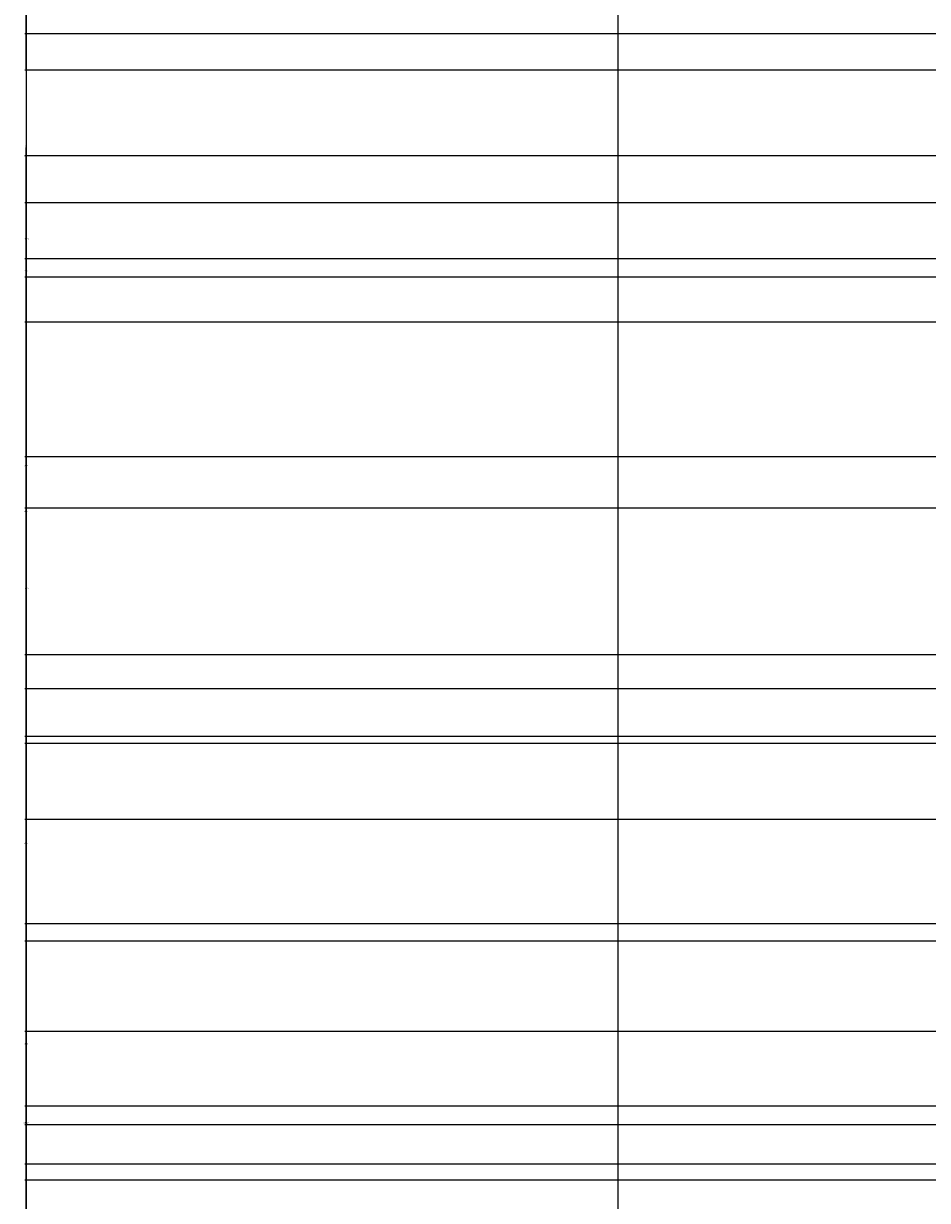
# Model space of a CAD drawing. Units: inches. Extents: x 818 to 1898, y 976 to 2364.
# Tile 57 of 96: x 818 to 950, y 1873 to 2046. Entities that reach past the tile are written whole.
import ezdxf

# ---------------------------------------------------------------- set-up
doc = ezdxf.new("R2010")
doc.units = ezdxf.units.IN
doc.header["$LTSCALE"] = 5
doc.header["$MEASUREMENT"] = 0
doc.layers.add('A-ANNO-DIMS', color=2, linetype='Continuous', lineweight=18)
doc.styles.get("Standard").update_dxf_attribs({"font": 'arial.ttf'})
doc.dimstyles.get("Standard").update_dxf_attribs({"dimtxt": 0.18, "dimasz": 0.18, "dimexe": 0.18, "dimexo": 0.0625, "dimgap": 0.09, "dimtad": 0, "dimtih": 1, "dimtoh": 1, "dimdec": 4, "dimzin": 0, "dimdsep": 46, "dimtxsty": 'Standard', "dimcen": 0.09, "dimadec": 0, "dimazin": 0, "dimtfac": 1, "dimtdec": 4, "dimtofl": 0, "dimtmove": 0, "dimatfit": 3, "dimfxl": 1, "dimtolj": 1, "dimtzin": 0, "dimarcsym": 0})

# ---------------------------------------------------------------- blocks, each defined once
blk = doc.blocks.new('*D59')
at = {"layer": 'A-ANNO-DIMS', "color": 0, "lineweight": -2, "ltscale": 5, "transparency": 16777216}
for p, q in [((1251.64, 2300.39), (818.03, 2300.39)), ((818.21, 2300.21), (818.21, 1669.95)), ((818.21, 1039.32), (818.21, 1669.59)), ((896.05, 1039.14), (818.03, 1039.14))]:
    blk.add_line(p, q, dxfattribs=at)
at = {"layer": 'A-ANNO-DIMS', "color": 0, "ltscale": 5, "transparency": 16777216}
for points in [[(818.18, 2300.21), (818.24, 2300.21), (818.21, 2300.39)], [(818.18, 1039.32), (818.24, 1039.32), (818.21, 1039.14)]]:
    blk.add_solid(points, dxfattribs=at)
at = {"layer": 'Defpoints', "color": 0, "ltscale": 5, "transparency": 16777216}
for p in [(818.21, 2300.39), (1251.71, 2300.39), (896.11, 1039.14)]:
    blk.add_point(p, dxfattribs=at)
at = {"layer": 'A-ANNO-DIMS', "color": 0, "ltscale": 5, "transparency": 16777216, "insert": (818.21, 1669.77), "char_height": 0.18, "attachment_point": 5}
blk.add_mtext('\\A1;1261.2', dxfattribs=at)
blk = doc.blocks.new('*D60')
at = {"layer": 'A-ANNO-DIMS', "color": 0, "lineweight": -2, "ltscale": 5, "transparency": 16777216}
for p, q in [((992.66, 2294.22), (818.03, 2294.22)), ((818.21, 2294.04), (818.21, 1748.77)), ((818.21, 1203.14), (818.21, 1748.41)), ((992.66, 1202.96), (818.03, 1202.96))]:
    blk.add_line(p, q, dxfattribs=at)
at = {"layer": 'A-ANNO-DIMS', "color": 0, "ltscale": 5, "transparency": 16777216}
for points in [[(818.18, 2294.04), (818.24, 2294.04), (818.21, 2294.22)], [(818.18, 1203.14), (818.24, 1203.14), (818.21, 1202.96)]]:
    blk.add_solid(points, dxfattribs=at)
at = {"layer": 'Defpoints', "color": 0, "ltscale": 5, "transparency": 16777216}
for p in [(818.21, 2294.22), (992.73, 2294.22), (992.73, 1202.96)]:
    blk.add_point(p, dxfattribs=at)
at = {"layer": 'A-ANNO-DIMS', "color": 0, "ltscale": 5, "transparency": 16777216, "insert": (818.21, 1748.59), "char_height": 0.18, "attachment_point": 5}
blk.add_mtext('\\A1;1091.3', dxfattribs=at)
blk = doc.blocks.new('*D73')
at = {"layer": 'A-ANNO-DIMS', "color": 0, "lineweight": -2, "ltscale": 5, "transparency": 16777216}
for p, q in [((1590.66, 2011.08), (818.03, 2011.08)), ((818.21, 2010.9), (818.21, 1996.76)), ((818.21, 1982.26), (818.21, 1996.4)), ((1590.66, 1982.08), (818.03, 1982.08))]:
    blk.add_line(p, q, dxfattribs=at)
at = {"layer": 'A-ANNO-DIMS', "color": 0, "ltscale": 5, "transparency": 16777216}
for points in [[(818.18, 2010.9), (818.24, 2010.9), (818.21, 2011.08)], [(818.18, 1982.26), (818.24, 1982.26), (818.21, 1982.08)]]:
    blk.add_solid(points, dxfattribs=at)
at = {"layer": 'Defpoints', "color": 0, "ltscale": 5, "transparency": 16777216}
for p in [(818.21, 2011.08), (1590.73, 2011.08), (1590.73, 1982.08)]:
    blk.add_point(p, dxfattribs=at)
at = {"layer": 'A-ANNO-DIMS', "color": 0, "ltscale": 5, "transparency": 16777216, "insert": (818.21, 1996.58), "char_height": 0.18, "attachment_point": 5}
blk.add_mtext('\\A1;29', dxfattribs=at)
blk = doc.blocks.new('*D74')
at = {"layer": 'A-ANNO-DIMS', "color": 0, "lineweight": -2, "ltscale": 5, "transparency": 16777216}
for p, q in [((1590.66, 1940.08), (818.03, 1940.08)), ((818.21, 1939.9), (818.21, 1925.76)), ((818.21, 1911.26), (818.21, 1925.4)), ((1590.66, 1911.08), (818.03, 1911.08))]:
    blk.add_line(p, q, dxfattribs=at)
at = {"layer": 'A-ANNO-DIMS', "color": 0, "ltscale": 5, "transparency": 16777216}
for points in [[(818.18, 1939.9), (818.24, 1939.9), (818.21, 1940.08)], [(818.18, 1911.26), (818.24, 1911.26), (818.21, 1911.08)]]:
    blk.add_solid(points, dxfattribs=at)
at = {"layer": 'Defpoints', "color": 0, "ltscale": 5, "transparency": 16777216}
for p in [(818.21, 1940.08), (1590.73, 1940.08), (1590.73, 1911.08)]:
    blk.add_point(p, dxfattribs=at)
at = {"layer": 'A-ANNO-DIMS', "color": 0, "ltscale": 5, "transparency": 16777216, "insert": (818.21, 1925.58), "char_height": 0.18, "attachment_point": 5}
blk.add_mtext('\\A1;29', dxfattribs=at)
blk = doc.blocks.new('*D90')
at = {"layer": 'A-ANNO-DIMS', "color": 0, "lineweight": -2, "ltscale": 5, "transparency": 16777216}
for p, q in [((904.95, 1071.12), (904.95, 2363.87)), ((905.13, 2363.69), (931.67, 2363.69)), ((958.99, 2363.69), (932.45, 2363.69)), ((959.17, 1071.12), (959.17, 2363.87))]:
    blk.add_line(p, q, dxfattribs=at)
at = {"layer": 'A-ANNO-DIMS', "color": 0, "ltscale": 5, "transparency": 16777216}
for points in [[(905.13, 2363.72), (905.13, 2363.66), (904.95, 2363.69)], [(958.99, 2363.72), (958.99, 2363.66), (959.17, 2363.69)]]:
    blk.add_solid(points, dxfattribs=at)
at = {"layer": 'Defpoints', "color": 0, "ltscale": 5, "transparency": 16777216}
for p in [(959.17, 2363.69), (904.95, 1071.06), (959.17, 1071.06)]:
    blk.add_point(p, dxfattribs=at)
at = {"layer": 'A-ANNO-DIMS', "color": 0, "ltscale": 5, "transparency": 16777216, "insert": (932.06, 2363.69), "char_height": 0.18, "attachment_point": 5}
blk.add_mtext('\\A1;54.22', dxfattribs=at)
blk = doc.blocks.new('*D121')
at = {"layer": 'A-ANNO-DIMS', "color": 0, "lineweight": -2, "ltscale": 5, "transparency": 16777216}
for p, q in [((1766.29, 1884.2), (818.03, 1884.2)), ((818.21, 1884.02), (818.21, 1841.14)), ((818.21, 1797.9), (818.21, 1840.78)), ((1766.29, 1797.72), (818.03, 1797.72))]:
    blk.add_line(p, q, dxfattribs=at)
at = {"layer": 'A-ANNO-DIMS', "color": 0, "ltscale": 5, "transparency": 16777216}
for points in [[(818.18, 1884.02), (818.24, 1884.02), (818.21, 1884.2)], [(818.18, 1797.9), (818.24, 1797.9), (818.21, 1797.72)]]:
    blk.add_solid(points, dxfattribs=at)
at = {"layer": 'Defpoints', "color": 0, "ltscale": 5, "transparency": 16777216}
for p in [(818.21, 1884.2), (1766.35, 1884.2), (1766.35, 1797.72)]:
    blk.add_point(p, dxfattribs=at)
at = {"layer": 'A-ANNO-DIMS', "color": 0, "ltscale": 5, "transparency": 16777216, "insert": (818.21, 1840.96), "char_height": 0.18, "attachment_point": 5}
blk.add_mtext('\\A1;86.49', dxfattribs=at)
blk = doc.blocks.new('*D124')
at = {"layer": 'A-ANNO-DIMS', "color": 0, "lineweight": -2, "ltscale": 5, "transparency": 16777216}
for p, q in [((1131.7, 1974.57), (818.03, 1974.57)), ((818.21, 1974.39), (818.21, 1884.68)), ((818.21, 1794.61), (818.21, 1884.32)), ((1138.44, 1794.43), (818.03, 1794.43))]:
    blk.add_line(p, q, dxfattribs=at)
at = {"layer": 'A-ANNO-DIMS', "color": 0, "ltscale": 5, "transparency": 16777216}
for points in [[(818.18, 1974.39), (818.24, 1974.39), (818.21, 1974.57)], [(818.18, 1794.61), (818.24, 1794.61), (818.21, 1794.43)]]:
    blk.add_solid(points, dxfattribs=at)
at = {"layer": 'Defpoints', "color": 0, "ltscale": 5, "transparency": 16777216}
for p in [(818.21, 1974.57), (1131.77, 1974.57), (1138.5, 1794.43)]:
    blk.add_point(p, dxfattribs=at)
at = {"layer": 'A-ANNO-DIMS', "color": 0, "ltscale": 5, "transparency": 16777216, "insert": (818.21, 1884.5), "char_height": 0.18, "attachment_point": 5}
blk.add_mtext('\\A1;180.14', dxfattribs=at)
blk = doc.blocks.new('*D125')
at = {"layer": 'A-ANNO-DIMS', "color": 0, "lineweight": -2, "ltscale": 5, "transparency": 16777216}
for p, q in [((1083.66, 2044.08), (818.03, 2044.08)), ((818.21, 2043.9), (818.21, 2009.51)), ((818.21, 1974.75), (818.21, 2009.14)), ((1131.7, 1974.57), (818.03, 1974.57))]:
    blk.add_line(p, q, dxfattribs=at)
at = {"layer": 'A-ANNO-DIMS', "color": 0, "ltscale": 5, "transparency": 16777216}
for points in [[(818.18, 2043.9), (818.24, 2043.9), (818.21, 2044.08)], [(818.18, 1974.75), (818.24, 1974.75), (818.21, 1974.57)]]:
    blk.add_solid(points, dxfattribs=at)
at = {"layer": 'Defpoints', "color": 0, "ltscale": 5, "transparency": 16777216}
for p in [(1083.73, 2044.08), (818.21, 1974.57), (1131.77, 1974.57)]:
    blk.add_point(p, dxfattribs=at)
at = {"layer": 'A-ANNO-DIMS', "color": 0, "ltscale": 5, "transparency": 16777216, "insert": (818.21, 2009.33), "char_height": 0.18, "attachment_point": 5}
blk.add_mtext('\\A1;69.5', dxfattribs=at)
blk = doc.blocks.new('*D131')
at = {"layer": 'A-ANNO-DIMS', "color": 0, "lineweight": -2, "ltscale": 5, "transparency": 16777216}
for p, q in [((1043.71, 1886.9), (818.03, 1886.9)), ((818.21, 1886.72), (818.21, 1805.95)), ((818.21, 1724.81), (818.21, 1805.58)), ((1044.78, 1724.63), (818.03, 1724.63))]:
    blk.add_line(p, q, dxfattribs=at)
at = {"layer": 'A-ANNO-DIMS', "color": 0, "ltscale": 5, "transparency": 16777216}
for points in [[(818.18, 1886.72), (818.24, 1886.72), (818.21, 1886.9)], [(818.18, 1724.81), (818.24, 1724.81), (818.21, 1724.63)]]:
    blk.add_solid(points, dxfattribs=at)
at = {"layer": 'Defpoints', "color": 0, "ltscale": 5, "transparency": 16777216}
for p in [(818.21, 1886.9), (1043.77, 1886.9), (1044.85, 1724.63)]:
    blk.add_point(p, dxfattribs=at)
at = {"layer": 'A-ANNO-DIMS', "color": 0, "ltscale": 5, "transparency": 16777216, "insert": (818.21, 1805.77), "char_height": 0.18, "attachment_point": 5}
blk.add_mtext('\\A1;162.27', dxfattribs=at)
blk = doc.blocks.new('*D132')
at = {"layer": 'A-ANNO-DIMS', "color": 0, "lineweight": -2, "ltscale": 5, "transparency": 16777216}
for p, q in [((1043.71, 2038.76), (818.03, 2038.76)), ((818.21, 2038.58), (818.21, 1963.01)), ((818.21, 1887.08), (818.21, 1962.65)), ((1043.71, 1886.9), (818.03, 1886.9))]:
    blk.add_line(p, q, dxfattribs=at)
at = {"layer": 'A-ANNO-DIMS', "color": 0, "ltscale": 5, "transparency": 16777216}
for points in [[(818.18, 2038.58), (818.24, 2038.58), (818.21, 2038.76)], [(818.18, 1887.08), (818.24, 1887.08), (818.21, 1886.9)]]:
    blk.add_solid(points, dxfattribs=at)
at = {"layer": 'Defpoints', "color": 0, "ltscale": 5, "transparency": 16777216}
for p in [(818.21, 2038.76), (1043.77, 2038.76), (1043.77, 1886.9)]:
    blk.add_point(p, dxfattribs=at)
at = {"layer": 'A-ANNO-DIMS', "color": 0, "ltscale": 5, "transparency": 16777216, "insert": (818.21, 1962.83), "char_height": 0.18, "attachment_point": 5}
blk.add_mtext('\\A1;151.86', dxfattribs=at)
blk = doc.blocks.new('*D133')
at = {"layer": 'A-ANNO-DIMS', "color": 0, "lineweight": -2, "ltscale": 5, "transparency": 16777216}
for p, q in [((1041.64, 2162.89), (818.03, 2162.89)), ((818.21, 2162.71), (818.21, 2101.01)), ((818.21, 2038.94), (818.21, 2100.64)), ((1043.71, 2038.76), (818.03, 2038.76))]:
    blk.add_line(p, q, dxfattribs=at)
at = {"layer": 'A-ANNO-DIMS', "color": 0, "ltscale": 5, "transparency": 16777216}
for points in [[(818.18, 2162.71), (818.24, 2162.71), (818.21, 2162.89)], [(818.18, 2038.94), (818.24, 2038.94), (818.21, 2038.76)]]:
    blk.add_solid(points, dxfattribs=at)
at = {"layer": 'Defpoints', "color": 0, "ltscale": 5, "transparency": 16777216}
for p in [(818.21, 2162.89), (1041.7, 2162.89), (1043.77, 2038.76)]:
    blk.add_point(p, dxfattribs=at)
at = {"layer": 'A-ANNO-DIMS', "color": 0, "ltscale": 5, "transparency": 16777216, "insert": (818.21, 2100.82), "char_height": 0.18, "attachment_point": 5}
blk.add_mtext('\\A1;124.13', dxfattribs=at)
blk = doc.blocks.new('*D162')
at = {"layer": 'A-ANNO-DIMS', "color": 0, "lineweight": -2, "ltscale": 5, "transparency": 16777216}
for p, q in [((1429.16, 1876.08), (818.03, 1876.08)), ((818.21, 1875.9), (818.21, 1871.76)), ((818.21, 1867.26), (818.21, 1871.4)), ((1429.16, 1867.08), (818.03, 1867.08))]:
    blk.add_line(p, q, dxfattribs=at)
at = {"layer": 'A-ANNO-DIMS', "color": 0, "ltscale": 5, "transparency": 16777216}
for points in [[(818.18, 1875.9), (818.24, 1875.9), (818.21, 1876.08)], [(818.18, 1867.26), (818.24, 1867.26), (818.21, 1867.08)]]:
    blk.add_solid(points, dxfattribs=at)
at = {"layer": 'Defpoints', "color": 0, "ltscale": 5, "transparency": 16777216}
for p in [(1429.23, 1876.08), (818.21, 1867.08), (1429.23, 1867.08)]:
    blk.add_point(p, dxfattribs=at)
at = {"layer": 'A-ANNO-DIMS', "color": 0, "ltscale": 5, "transparency": 16777216, "insert": (818.21, 1871.58), "char_height": 0.18, "attachment_point": 5}
blk.add_mtext('\\A1;9', dxfattribs=at)
blk = doc.blocks.new('*D206')
at = {"layer": 'A-ANNO-DIMS', "color": 0, "lineweight": -2, "ltscale": 5, "transparency": 16777216}
for p, q in [((1590.66, 1911.08), (818.03, 1911.08)), ((818.21, 1910.9), (818.21, 1893.76)), ((818.21, 1876.26), (818.21, 1893.4)), ((1590.66, 1876.08), (818.03, 1876.08))]:
    blk.add_line(p, q, dxfattribs=at)
at = {"layer": 'A-ANNO-DIMS', "color": 0, "ltscale": 5, "transparency": 16777216}
for points in [[(818.18, 1910.9), (818.24, 1910.9), (818.21, 1911.08)], [(818.18, 1876.26), (818.24, 1876.26), (818.21, 1876.08)]]:
    blk.add_solid(points, dxfattribs=at)
at = {"layer": 'Defpoints', "color": 0, "ltscale": 5, "transparency": 16777216}
for p in [(818.21, 1911.08), (1590.73, 1911.08), (1590.73, 1876.08)]:
    blk.add_point(p, dxfattribs=at)
at = {"layer": 'A-ANNO-DIMS', "color": 0, "ltscale": 5, "transparency": 16777216, "insert": (818.21, 1893.58), "char_height": 0.18, "attachment_point": 5}
blk.add_mtext('\\A1;35', dxfattribs=at)
blk = doc.blocks.new('*D207')
at = {"layer": 'A-ANNO-DIMS', "color": 0, "lineweight": -2, "ltscale": 5, "transparency": 16777216}
for p, q in [((1590.66, 2044.08), (818.03, 2044.08)), ((818.21, 2043.9), (818.21, 2027.76)), ((818.21, 2011.26), (818.21, 2027.4)), ((1590.66, 2011.08), (818.03, 2011.08))]:
    blk.add_line(p, q, dxfattribs=at)
at = {"layer": 'A-ANNO-DIMS', "color": 0, "ltscale": 5, "transparency": 16777216}
for points in [[(818.18, 2043.9), (818.24, 2043.9), (818.21, 2044.08)], [(818.18, 2011.26), (818.24, 2011.26), (818.21, 2011.08)]]:
    blk.add_solid(points, dxfattribs=at)
at = {"layer": 'Defpoints', "color": 0, "ltscale": 5, "transparency": 16777216}
for p in [(818.21, 2044.08), (1590.73, 2044.08), (1590.73, 2011.08)]:
    blk.add_point(p, dxfattribs=at)
at = {"layer": 'A-ANNO-DIMS', "color": 0, "ltscale": 5, "transparency": 16777216, "insert": (818.21, 2027.58), "char_height": 0.18, "attachment_point": 5}
blk.add_mtext('\\A1;33', dxfattribs=at)
blk = doc.blocks.new('*D211')
at = {"layer": 'A-ANNO-DIMS', "color": 0, "lineweight": -2, "ltscale": 5, "transparency": 16777216}
for p, q in [((1599.66265, 1948.078237), (818.025912, 1948.078237)), ((818.205912, 1947.898237), (818.205912, 1944.758237)), ((818.205912, 1941.258237), (818.205912, 1944.398237)), ((1599.66265, 1941.078237), (818.025912, 1941.078237))]:
    blk.add_line(p, q, dxfattribs=at)
at = {"layer": 'A-ANNO-DIMS', "color": 0, "ltscale": 5, "transparency": 16777216}
for points in [[(818.175912, 1947.898237), (818.235912, 1947.898237), (818.205912, 1948.078237)], [(818.175912, 1941.258237), (818.235912, 1941.258237), (818.205912, 1941.078237)]]:
    blk.add_solid(points, dxfattribs=at)
at = {"layer": 'Defpoints', "color": 0, "ltscale": 5, "transparency": 16777216}
for p in [(818.205912, 1948.078237), (1599.72515, 1948.078237), (1599.72515, 1941.078237)]:
    blk.add_point(p, dxfattribs=at)
at = {"layer": 'A-ANNO-DIMS', "color": 0, "ltscale": 5, "transparency": 16777216, "insert": (818.205912, 1944.578237), "char_height": 0.18, "attachment_point": 5}
blk.add_mtext('\\A1;7', dxfattribs=at)
blk = doc.blocks.new('*D215')
at = {"layer": 'A-ANNO-DIMS', "color": 0, "lineweight": -2, "ltscale": 5, "transparency": 16777216}
for p, q in [((1590.66, 1876.08), (818.03, 1876.08)), ((818.21, 1875.9), (818.21, 1781.76)), ((818.21, 1687.26), (818.21, 1781.4)), ((1511.66, 1687.08), (818.03, 1687.08))]:
    blk.add_line(p, q, dxfattribs=at)
at = {"layer": 'A-ANNO-DIMS', "color": 0, "ltscale": 5, "transparency": 16777216}
for points in [[(818.18, 1875.9), (818.24, 1875.9), (818.21, 1876.08)], [(818.18, 1687.26), (818.24, 1687.26), (818.21, 1687.08)]]:
    blk.add_solid(points, dxfattribs=at)
at = {"layer": 'Defpoints', "color": 0, "ltscale": 5, "transparency": 16777216}
for p in [(818.21, 1876.08), (1590.73, 1876.08), (1511.73, 1687.08)]:
    blk.add_point(p, dxfattribs=at)
at = {"layer": 'A-ANNO-DIMS', "color": 0, "ltscale": 5, "transparency": 16777216, "insert": (818.21, 1781.58), "char_height": 0.18, "attachment_point": 5}
blk.add_mtext('\\A1;189', dxfattribs=at)
blk = doc.blocks.new('*D232')
at = {"layer": 'A-ANNO-DIMS', "color": 0, "lineweight": -2, "ltscale": 5, "transparency": 16777216}
for p, q in [((1303.87, 2008.39), (818.03, 2008.39)), ((818.21, 2008.21), (818.21, 1980.9)), ((818.21, 1953.22), (818.21, 1980.53)), ((1303.87, 1953.04), (818.03, 1953.04))]:
    blk.add_line(p, q, dxfattribs=at)
at = {"layer": 'A-ANNO-DIMS', "color": 0, "ltscale": 5, "transparency": 16777216}
for points in [[(818.18, 2008.21), (818.24, 2008.21), (818.21, 2008.39)], [(818.18, 1953.22), (818.24, 1953.22), (818.21, 1953.04)]]:
    blk.add_solid(points, dxfattribs=at)
at = {"layer": 'Defpoints', "color": 0, "ltscale": 5, "transparency": 16777216}
for p in [(818.21, 2008.39), (1303.93, 2008.39), (1303.93, 1953.04)]:
    blk.add_point(p, dxfattribs=at)
at = {"layer": 'A-ANNO-DIMS', "color": 0, "ltscale": 5, "transparency": 16777216, "insert": (818.21, 1980.72), "char_height": 0.18, "attachment_point": 5}
blk.add_mtext('\\A1;55.35', dxfattribs=at)
blk = doc.blocks.new('*D234')
at = {"layer": 'A-ANNO-DIMS', "color": 0, "lineweight": -2, "ltscale": 5, "transparency": 16777216}
for p, q in [((1267.66, 2044.08), (818.03, 2044.08)), ((818.21, 2043.9), (818.21, 2026.42)), ((818.21, 2008.57), (818.21, 2026.05)), ((1303.87, 2008.39), (818.03, 2008.39))]:
    blk.add_line(p, q, dxfattribs=at)
at = {"layer": 'A-ANNO-DIMS', "color": 0, "ltscale": 5, "transparency": 16777216}
for points in [[(818.18, 2043.9), (818.24, 2043.9), (818.21, 2044.08)], [(818.18, 2008.57), (818.24, 2008.57), (818.21, 2008.39)]]:
    blk.add_solid(points, dxfattribs=at)
at = {"layer": 'Defpoints', "color": 0, "ltscale": 5, "transparency": 16777216}
for p in [(818.21, 2044.08), (1267.73, 2044.08), (1303.93, 2008.39)]:
    blk.add_point(p, dxfattribs=at)
at = {"layer": 'A-ANNO-DIMS', "color": 0, "ltscale": 5, "transparency": 16777216, "insert": (818.21, 2026.23), "char_height": 0.18, "attachment_point": 5}
blk.add_mtext('\\A1;35.69', dxfattribs=at)
blk = doc.blocks.new('*D237')
at = {"layer": 'A-ANNO-DIMS', "color": 0, "lineweight": -2, "ltscale": 5, "transparency": 16777216}
for p, q in [((1310.85, 2026.21), (818.03, 2026.21)), ((818.21, 2026.03), (818.21, 2014.2)), ((818.21, 2002), (818.21, 2013.83)), ((1314.2, 2001.82), (818.03, 2001.82))]:
    blk.add_line(p, q, dxfattribs=at)
at = {"layer": 'A-ANNO-DIMS', "color": 0, "ltscale": 5, "transparency": 16777216}
for points in [[(818.18, 2026.03), (818.24, 2026.03), (818.21, 2026.21)], [(818.18, 2002), (818.24, 2002), (818.21, 2001.82)]]:
    blk.add_solid(points, dxfattribs=at)
at = {"layer": 'Defpoints', "color": 0, "ltscale": 5, "transparency": 16777216}
for p in [(1310.91, 2026.21), (818.21, 2001.82), (1314.26, 2001.82)]:
    blk.add_point(p, dxfattribs=at)
at = {"layer": 'A-ANNO-DIMS', "color": 0, "ltscale": 5, "transparency": 16777216, "insert": (818.21, 2014.02), "char_height": 0.18, "attachment_point": 5}
blk.add_mtext('\\A1;24.383', dxfattribs=at)
blk = doc.blocks.new('*D248')
at = {"layer": 'A-ANNO-DIMS', "color": 0, "lineweight": -2, "ltscale": 5, "transparency": 16777216}
for p, q in [((1258.66, 2019.29), (818.03, 2019.29)), ((818.21, 2019.11), (818.21, 1974.29)), ((818.21, 1929.1), (818.21, 1973.92)), ((1258.66, 1928.92), (818.03, 1928.92))]:
    blk.add_line(p, q, dxfattribs=at)
at = {"layer": 'A-ANNO-DIMS', "color": 0, "ltscale": 5, "transparency": 16777216}
for points in [[(818.18, 2019.11), (818.24, 2019.11), (818.21, 2019.29)], [(818.18, 1929.1), (818.24, 1929.1), (818.21, 1928.92)]]:
    blk.add_solid(points, dxfattribs=at)
at = {"layer": 'Defpoints', "color": 0, "ltscale": 5, "transparency": 16777216}
for p in [(818.21, 2019.29), (1258.73, 2019.29), (1258.73, 1928.92)]:
    blk.add_point(p, dxfattribs=at)
at = {"layer": 'A-ANNO-DIMS', "color": 0, "ltscale": 5, "transparency": 16777216, "insert": (818.21, 1974.1), "char_height": 0.18, "attachment_point": 5}
blk.add_mtext('\\A1;90.37', dxfattribs=at)
blk = doc.blocks.new('*D250')
at = {"layer": 'A-ANNO-DIMS', "color": 0, "lineweight": -2, "ltscale": 5, "transparency": 16777216}
for p, q in [((1250.24, 1913.64), (818.03, 1913.64)), ((818.21, 1913.46), (818.21, 1896.2)), ((818.21, 1878.57), (818.21, 1895.83)), ((1250.24, 1878.39), (818.03, 1878.39))]:
    blk.add_line(p, q, dxfattribs=at)
at = {"layer": 'A-ANNO-DIMS', "color": 0, "ltscale": 5, "transparency": 16777216}
for points in [[(818.18, 1913.46), (818.24, 1913.46), (818.21, 1913.64)], [(818.18, 1878.57), (818.24, 1878.57), (818.21, 1878.39)]]:
    blk.add_solid(points, dxfattribs=at)
at = {"layer": 'Defpoints', "color": 0, "ltscale": 5, "transparency": 16777216}
for p in [(818.21, 1913.64), (1250.3, 1913.64), (1250.3, 1878.39)]:
    blk.add_point(p, dxfattribs=at)
at = {"layer": 'A-ANNO-DIMS', "color": 0, "ltscale": 5, "transparency": 16777216, "insert": (818.21, 1896.02), "char_height": 0.18, "attachment_point": 5}
blk.add_mtext('\\A1;35.25', dxfattribs=at)
blk = doc.blocks.new('*D287')
at = {"layer": 'A-ANNO-DIMS', "color": 0, "lineweight": -2, "ltscale": 5, "transparency": 16777216}
for p, q in [((1303.87, 1953.04), (818.03, 1953.04)), ((818.21, 1952.86), (818.21, 1925.64)), ((818.21, 1898.05), (818.21, 1925.27)), ((1310.96, 1897.87), (818.03, 1897.87))]:
    blk.add_line(p, q, dxfattribs=at)
at = {"layer": 'A-ANNO-DIMS', "color": 0, "ltscale": 5, "transparency": 16777216}
for points in [[(818.18, 1952.86), (818.24, 1952.86), (818.21, 1953.04)], [(818.18, 1898.05), (818.24, 1898.05), (818.21, 1897.87)]]:
    blk.add_solid(points, dxfattribs=at)
at = {"layer": 'Defpoints', "color": 0, "ltscale": 5, "transparency": 16777216}
for p in [(818.21, 1953.04), (1303.93, 1953.04), (1311.03, 1897.87)]:
    blk.add_point(p, dxfattribs=at)
at = {"layer": 'A-ANNO-DIMS', "color": 0, "ltscale": 5, "transparency": 16777216, "insert": (818.21, 1925.45), "char_height": 0.18, "attachment_point": 5}
blk.add_mtext('\\A1;55.17', dxfattribs=at)

msp = doc.modelspace()

# ---------------------------------------------------------------- dimensions: what is measured, and where the dimension line sits
at = {"layer": 'A-ANNO-DIMS', "ltscale": 5}
dim = msp.add_linear_dim(base=(959.1737, 2363.6929), p1=(904.9504, 1071.0552), p2=(959.1737, 1071.0552), dimstyle='Standard', override={"dimdec": 2, "dimlfac": 1, "dimrnd": 0, "dimzin": 0, "dimdsep": 46, "dimlunit": 2}, dxfattribs=at)
dim.commit()
dim.dimension.update_dxf_attribs({"geometry": '*D90', "text_midpoint": (932.062, 2363.6929)})
for base, p1, p2, override, picture, middle in [((818.2059, 2300.3929), (896.1138, 1039.1433), (1251.7057, 2300.3929), {"dimdec": 1, "dimlfac": 1, "dimrnd": 0, "dimzin": 0, "dimdsep": 46, "dimlunit": 2}, '*D59', (818.2059, 1669.7681)), ((818.2059, 2294.2171), (992.7251, 1202.9642), (992.7251, 2294.2171), {"dimdec": 1, "dimlfac": 1, "dimrnd": 0, "dimzin": 0, "dimdsep": 46, "dimlunit": 2}, '*D60', (818.2059, 1748.5907)), ((818.2059, 2162.8898), (1043.7685, 2038.7583), (1041.7008, 2162.8898), {"dimdec": 2, "dimlfac": 1, "dimrnd": 0, "dimzin": 0, "dimdsep": 46, "dimlunit": 2}, '*D133', (818.2059, 2100.824)), ((818.2059, 2044.0782), (1303.9314, 2008.3917), (1267.7251, 2044.0782), {"dimdec": 2, "dimlfac": 1, "dimrnd": 0, "dimzin": 0, "dimdsep": 46, "dimlunit": 2}, '*D234', (818.2059, 2026.235)), ((818.2059, 1974.5735), (1083.7251, 2044.0782), (1131.7651, 1974.5735), {"dimdec": 1, "dimlfac": 1, "dimrnd": 0, "dimzin": 0, "dimdsep": 46, "dimlunit": 2}, '*D125', (818.2059, 2009.3258)), ((818.2059, 2044.0782), (1590.7251, 2011.0782), (1590.7251, 2044.0782), {"dimdec": 0, "dimlfac": 1, "dimrnd": 0, "dimzin": 0, "dimdsep": 46, "dimlunit": 2}, '*D207', (818.2059, 2027.5782)), ((818.2059, 2038.7583), (1043.7685, 1886.9018), (1043.7685, 2038.7583), {"dimdec": 2, "dimlfac": 1, "dimrnd": 0, "dimzin": 0, "dimdsep": 46, "dimlunit": 2}, '*D132', (818.2059, 1962.83)), ((818.2059, 2001.8247), (1310.9077, 2026.2074), (1314.2595, 2001.8247), {"dimdec": 3, "dimlfac": 1, "dimrnd": 0, "dimzin": 0, "dimdsep": 46, "dimlunit": 2}, '*D237', (818.2059, 2014.016)), ((818.2059, 2019.2871), (1258.7251, 1928.9218), (1258.7251, 2019.2871), {"dimdec": 2, "dimlfac": 1, "dimrnd": 0, "dimzin": 0, "dimdsep": 46, "dimlunit": 2}, '*D248', (818.2059, 1974.1044)), ((818.2059, 2011.0782), (1590.7251, 1982.0782), (1590.7251, 2011.0782), {"dimdec": 0, "dimlfac": 1, "dimrnd": 0, "dimzin": 0, "dimdsep": 46, "dimlunit": 2}, '*D73', (818.2059, 1996.5782)), ((818.2059, 2008.3917), (1303.9314, 1953.0408), (1303.9314, 2008.3917), {"dimdec": 2, "dimlfac": 1, "dimrnd": 0, "dimzin": 0, "dimdsep": 46, "dimlunit": 2}, '*D232', (818.2059, 1980.7163)), ((818.2059, 1974.5735), (1138.5041, 1794.4325), (1131.7651, 1974.5735), {"dimdec": 2, "dimlfac": 1, "dimrnd": 0, "dimzin": 0, "dimdsep": 46, "dimlunit": 2}, '*D124', (818.2059, 1884.503)), ((818.2059, 1953.0408), (1311.025, 1897.8663), (1303.9314, 1953.0408), {"dimdec": 2, "dimlfac": 1, "dimrnd": 0, "dimzin": 0, "dimdsep": 46, "dimlunit": 2}, '*D287', (818.2059, 1925.4536)), ((818.2059, 1948.0782), (1599.7251, 1941.0782), (1599.7251, 1948.0782), {"dimdec": 0, "dimlfac": 1, "dimrnd": 0, "dimzin": 0, "dimdsep": 46, "dimlunit": 2}, '*D211', (818.2059, 1944.5782)), ((818.2059, 1940.0782), (1590.7251, 1911.0782), (1590.7251, 1940.0782), {"dimdec": 0, "dimlfac": 1, "dimrnd": 0, "dimzin": 0, "dimdsep": 46, "dimlunit": 2}, '*D74', (818.2059, 1925.5782)), ((818.2059, 1913.6401), (1250.3029, 1878.3919), (1250.3029, 1913.6401), {"dimdec": 2, "dimlfac": 1, "dimrnd": 0, "dimzin": 0, "dimdsep": 46, "dimlunit": 2}, '*D250', (818.2059, 1896.016)), ((818.2059, 1911.0782), (1590.7251, 1876.0782), (1590.7251, 1911.0782), {"dimdec": 0, "dimlfac": 1, "dimrnd": 0, "dimzin": 0, "dimdsep": 46, "dimlunit": 2}, '*D206', (818.2059, 1893.5782)), ((818.2059, 1886.9018), (1044.8463, 1724.63), (1043.7685, 1886.9018), {"dimdec": 2, "dimlfac": 1, "dimrnd": 0, "dimzin": 0, "dimdsep": 46, "dimlunit": 2}, '*D131', (818.2059, 1805.7659)), ((818.2059, 1884.2031), (1766.3524, 1797.7165), (1766.3524, 1884.2031), {"dimdec": 2, "dimlfac": 1, "dimrnd": 0, "dimzin": 0, "dimdsep": 46, "dimlunit": 2}, '*D121', (818.2059, 1840.9598)), ((818.2059, 1876.0782), (1511.7251, 1687.0782), (1590.7251, 1876.0782), {"dimdec": 0, "dimlfac": 1, "dimrnd": 0, "dimzin": 0, "dimdsep": 46, "dimlunit": 2}, '*D215', (818.2059, 1781.5782)), ((818.2059, 1867.0782), (1429.2251, 1876.0782), (1429.2251, 1867.0782), {"dimdec": 0, "dimlfac": 1, "dimrnd": 0, "dimzin": 0, "dimdsep": 46, "dimlunit": 2}, '*D162', (818.2059, 1871.5782))]:
    dim = msp.add_linear_dim(base=base, p1=p1, p2=p2, angle=90, dimstyle='Standard', override=override, dxfattribs=at)
    dim.commit()
    dim.dimension.update_dxf_attribs({"geometry": picture, "text_midpoint": middle})

doc.saveas('drawing.dxf')
